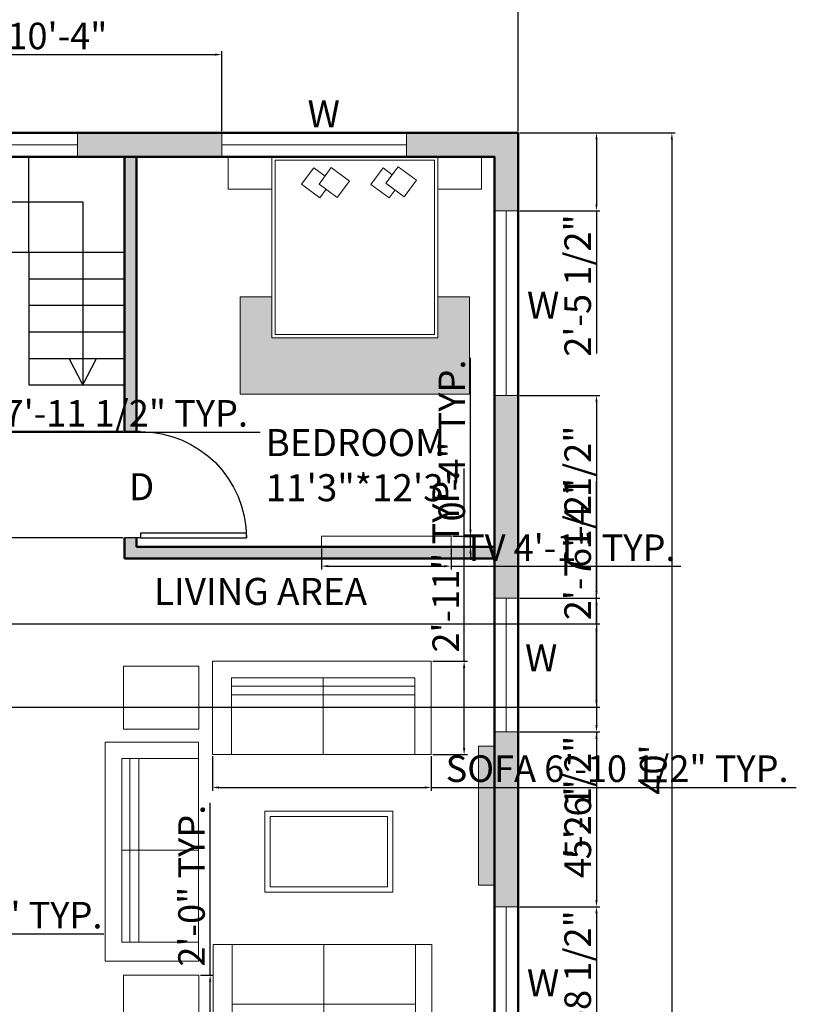
# Model space of a CAD drawing. Units: inches. Extents: x 1822 to 2392, y 2066 to 2908.
# Tile 3 of 4: x 2080 to 2373, y 2256 to 2627. Entities that reach past the tile are written whole.
import ezdxf

# ---------------------------------------------------------------- set-up
doc = ezdxf.new("R2010")
doc.units = ezdxf.units.IN
for name, color, linetype, lineweight in [('A-ANNO-DIMS', 2, 'Continuous', 18), ('A-AREA-IDEN', 83, 'Continuous', 25), ('A-EQPM-PATT', 89, 'Continuous', 13), ('A-FLOR-PATT', 9, 'Continuous', 13), ('A-FURN', 140, 'Continuous', 18), ('A-WALL-PATT', 252, 'Continuous', 13), ('BEDS', 40, 'Continuous', 18), ('DOOR', 50, 'Continuous', 25), ('SOFA', 140, 'Continuous', 18), ('STAIR', 32, 'Continuous', 25), ('TEXT', 83, 'Continuous', 25), ('TV', 89, 'Continuous', 18), ('wall', 7, 'Continuous', 50), ('WINDOW', 80, 'Continuous', 20)]:
    doc.layers.add(name, color=color, linetype=linetype, lineweight=lineweight)
doc.styles.get("Standard").update_dxf_attribs({"font": 'arial.ttf'})
doc.dimstyles.new('ISO-25', dxfattribs={"dimtxt": 10, "dimasz": 2.5, "dimexe": 1.25, "dimexo": 0.625, "dimtad": 1, "dimdec": 0, "dimlunit": 4, "dimtxsty": 'Standard', "dimcen": 2.5, "dimadec": 0, "dimazin": 0, "dimtfac": 1, "dimtdec": 0, "dimtmove": 0, "dimatfit": 3, "dimfxl": 1, "dimarcsym": 0})

# ---------------------------------------------------------------- blocks, each defined once
blk = doc.blocks.new('*U2')
for p, q in [((0, 0), (0, -6)), ((40, 0), (40, -6))]:
    blk.add_line(p, q)
blk.add_lwpolyline([(0, 0), (0, 40), (1.75, 40), (1.75, 0)], close=True)
blk.add_arc((0, 0), 40, 0, 90)
blk = doc.blocks.new('*D5')
at = {"layer": 'A-ANNO-DIMS', "color": 0, "lineweight": -2, "transparency": 16777216}
for p, q in [((1872.41, 2584.74), (1872.41, 2632.85)), ((1874.91, 2631.6), (2265.91, 2631.6)), ((2268.41, 2584.74), (2268.41, 2632.85))]:
    blk.add_line(p, q, dxfattribs=at)
at = {"layer": 'A-ANNO-DIMS', "color": 0, "transparency": 16777216}
for points in [[(1874.91, 2632.01), (1874.91, 2631.18), (1872.41, 2631.6)], [(2265.91, 2632.01), (2265.91, 2631.18), (2268.41, 2631.6)]]:
    blk.add_solid(points, dxfattribs=at)
at = {"layer": 'Defpoints', "color": 0, "transparency": 16777216}
for p in [(2268.41, 2631.6), (1872.41, 2584.12), (2268.41, 2584.12)]:
    blk.add_point(p, dxfattribs=at)
at = {"layer": 'A-ANNO-DIMS', "color": 0, "transparency": 16777216, "insert": (2070.41, 2637.33), "char_height": 10, "attachment_point": 5}
blk.add_mtext("33'", dxfattribs=at)
blk = doc.blocks.new('*D6')
at = {"layer": 'A-ANNO-DIMS', "color": 0, "lineweight": -2, "transparency": 16777216}
for p, q in [((2269.04, 2584.12), (2327.59, 2584.12)), ((2326.34, 2581.62), (2326.34, 2106.62)), ((2269.04, 2104.12), (2327.59, 2104.12))]:
    blk.add_line(p, q, dxfattribs=at)
at = {"layer": 'A-ANNO-DIMS', "color": 0, "transparency": 16777216}
for points in [[(2325.93, 2581.62), (2326.76, 2581.62), (2326.34, 2584.12)], [(2325.93, 2106.62), (2326.76, 2106.62), (2326.34, 2104.12)]]:
    blk.add_solid(points, dxfattribs=at)
at = {"layer": 'Defpoints', "color": 0, "transparency": 16777216}
for p in [(2268.41, 2584.12), (2268.41, 2104.12), (2326.34, 2104.12)]:
    blk.add_point(p, dxfattribs=at)
at = {"layer": 'A-ANNO-DIMS', "color": 0, "transparency": 16777216, "insert": (2320.61, 2344.12), "char_height": 10, "attachment_point": 5, "rotation": 90}
blk.add_mtext("40'", dxfattribs=at)
blk = doc.blocks.new('BED-DOUBLE-WITH-NIGHTSTANDS')
for p, q in [((0, -52.84), (-12, -52.84)), ((-12, -52.84), (-12, -89.47)), ((62.55, -52.84), (74.55, -52.84)), ((74.55, -52.84), (74.55, -89.47)), ((-12, -89.47), (74.55, -89.47))]:
    blk.add_line(p, q)
for points in [[(0, 0), (-16.5, 0), (-16.5, -12.19), (0, -12.19)], [(0, 0), (62.55, 0), (62.55, -68.27), (0, -68.27)], [(79.04, 0), (62.55, 0), (62.55, -12.19), (79.04, -12.19)], [(1.28, -1.28), (61.27, -1.28), (61.27, -67), (1.28, -67)], [(22.38, -4.1), (29.25, -9.19), (24.65, -15.4), (17.78, -10.31)], [(47.61, -3.78), (54.48, -8.87), (49.87, -15.08), (43, -9.99)]]:
    blk.add_lwpolyline(points, close=True)
for points in [[(20.42, -12.27), (18.06, -15.45), (11.2, -10.36), (15.8, -4.15), (20.02, -7.28)], [(46.41, -12.52), (44.19, -15.51), (37.32, -10.42), (41.93, -4.21), (45.39, -6.77)]]:
    blk.add_lwpolyline(points)
blk = doc.blocks.new('SOFA-TWO-SEAT')
for p, q in [((0, 0), (0, 35.2)), ((0, 35.2), (82.54, 35.2)), ((82.54, 35.2), (82.54, 0)), ((41.75, 28.9), (41.75, 0)), ((7.18, 25.83), (76.33, 25.83)), ((7.18, 22.51), (76.33, 22.51)), ((7.18, 0), (0, 0)), ((82.54, 0), (73.14, 0))]:
    blk.add_line(p, q)
blk.add_lwpolyline([(76.33, 0), (7.18, 0), (7.18, 28.9), (76.33, 28.9)], close=True)
blk = doc.blocks.new('WINDOW-EXT-TYPE-A')
blk.add_line((0, 4.5), (69.61, 4.5))
blk.add_lwpolyline([(0, 9), (69.61, 9), (69.61, 0), (0, 0)], close=True)
blk = doc.blocks.new('TABLE-END')
blk.add_lwpolyline([(0, 0), (28.42, 0), (28.42, 23.78), (0, 23.78)], close=True)
blk = doc.blocks.new('TV-BEDROOM-TYPE-A')
blk.add_lwpolyline([(0, 0), (48.81, 0), (48.81, 3.94), (0, 3.94)], close=True)
blk = doc.blocks.new('*D16')
at = {"layer": 'A-ANNO-DIMS', "color": 0, "lineweight": -2, "transparency": 16777216}
for p, q in [((1892.52, 2485.02), (1892.52, 2470.06)), ((1988.06, 2485.02), (1988.06, 2470.06)), ((1895.02, 2471.31), (1985.56, 2471.31)), ((1988.06, 2471.31), (2171.11, 2471.31))]:
    blk.add_line(p, q, dxfattribs=at)
at = {"layer": 'A-ANNO-DIMS', "color": 0, "transparency": 16777216}
for points in [[(1895.02, 2471.73), (1895.02, 2470.9), (1892.52, 2471.31)], [(1985.56, 2471.73), (1985.56, 2470.9), (1988.06, 2471.31)]]:
    blk.add_solid(points, dxfattribs=at)
at = {"layer": 'Defpoints', "color": 0, "transparency": 16777216}
for p in [(1892.52, 2485.65), (1988.06, 2485.65), (1988.06, 2471.31)]:
    blk.add_point(p, dxfattribs=at)
at = {"layer": 'A-ANNO-DIMS', "color": 0, "transparency": 16777216, "insert": (2080.84, 2477.11), "char_height": 10, "attachment_point": 5}
blk.add_mtext('BED GROUP 7\'-11 1/2" TYP.', dxfattribs=at)
blk = doc.blocks.new('*D18')
at = {"layer": 'A-ANNO-DIMS', "color": 0, "lineweight": -2, "transparency": 16777216}
for p, q in [((2153.07, 2349.12), (2153.07, 2336.11)), ((2235.61, 2349.12), (2235.61, 2336.11)), ((2155.57, 2337.36), (2233.11, 2337.36)), ((2235.61, 2337.36), (2373.26, 2337.36))]:
    blk.add_line(p, q, dxfattribs=at)
at = {"layer": 'A-ANNO-DIMS', "color": 0, "transparency": 16777216}
for points in [[(2155.57, 2337.78), (2155.57, 2336.95), (2153.07, 2337.36)], [(2233.11, 2337.78), (2233.11, 2336.95), (2235.61, 2337.36)]]:
    blk.add_solid(points, dxfattribs=at)
at = {"layer": 'Defpoints', "color": 0, "transparency": 16777216}
for p in [(2153.07, 2349.75), (2235.61, 2349.75), (2235.61, 2337.36)]:
    blk.add_point(p, dxfattribs=at)
at = {"layer": 'A-ANNO-DIMS', "color": 0, "transparency": 16777216, "insert": (2305.69, 2343.16), "char_height": 10, "attachment_point": 5}
blk.add_mtext('SOFA 6\'-10 1/2" TYP.', dxfattribs=at)
blk = doc.blocks.new('*D19')
at = {"layer": 'A-ANNO-DIMS', "color": 0, "lineweight": -2, "transparency": 16777216}
for p, q in [((2248, 2384.94), (2248, 2457.59)), ((2236.24, 2384.94), (2249.25, 2384.94)), ((2248, 2352.25), (2248, 2382.44)), ((2236.24, 2349.75), (2249.25, 2349.75))]:
    blk.add_line(p, q, dxfattribs=at)
at = {"layer": 'A-ANNO-DIMS', "color": 0, "transparency": 16777216}
for points in [[(2247.58, 2382.44), (2248.41, 2382.44), (2248, 2384.94)], [(2247.58, 2352.25), (2248.41, 2352.25), (2248, 2349.75)]]:
    blk.add_solid(points, dxfattribs=at)
at = {"layer": 'Defpoints', "color": 0, "transparency": 16777216}
for p in [(2235.61, 2384.94), (2248, 2384.94), (2235.61, 2349.75)]:
    blk.add_point(p, dxfattribs=at)
at = {"layer": 'A-ANNO-DIMS', "color": 0, "transparency": 16777216, "insert": (2242.35, 2422.51), "char_height": 10, "attachment_point": 5, "rotation": 90}
blk.add_mtext('2\'-11" TYP.', dxfattribs=at)
blk = doc.blocks.new('*D23')
at = {"layer": 'A-ANNO-DIMS', "color": 0, "lineweight": -2, "transparency": 16777216}
for p, q in [((2004.74, 2284.62), (2004.74, 2280.89)), ((2016.41, 2284.62), (2016.41, 2280.89)), ((2007.24, 2282.14), (2013.91, 2282.14)), ((2016.41, 2282.14), (2112.19, 2282.14))]:
    blk.add_line(p, q, dxfattribs=at)
at = {"layer": 'A-ANNO-DIMS', "color": 0, "transparency": 16777216}
for points in [[(2007.24, 2282.56), (2007.24, 2281.73), (2004.74, 2282.14)], [(2013.91, 2282.56), (2013.91, 2281.73), (2016.41, 2282.14)]]:
    blk.add_solid(points, dxfattribs=at)
at = {"layer": 'Defpoints', "color": 0, "transparency": 16777216}
for p in [(2004.74, 2285.25), (2016.41, 2285.25), (2016.41, 2282.14)]:
    blk.add_point(p, dxfattribs=at)
at = {"layer": 'A-ANNO-DIMS', "color": 0, "transparency": 16777216, "insert": (2065.55, 2287.94), "char_height": 10, "attachment_point": 5}
blk.add_mtext('0\'-11 1/2" TYP.', dxfattribs=at)
blk = doc.blocks.new('*D24')
at = {"layer": 'A-ANNO-DIMS', "color": 0, "lineweight": -2, "transparency": 16777216}
for p, q in [((2119.55, 2242.25), (2119.55, 2237.36)), ((2147.97, 2242.25), (2147.97, 2237.36)), ((2122.05, 2238.61), (2145.47, 2238.61)), ((2147.97, 2238.61), (2316.96, 2238.61))]:
    blk.add_line(p, q, dxfattribs=at)
at = {"layer": 'A-ANNO-DIMS', "color": 0, "transparency": 16777216}
for points in [[(2122.05, 2239.03), (2122.05, 2238.2), (2119.55, 2238.61)], [(2145.47, 2239.03), (2145.47, 2238.2), (2147.97, 2238.61)]]:
    blk.add_solid(points, dxfattribs=at)
at = {"layer": 'Defpoints', "color": 0, "transparency": 16777216}
for p in [(2119.55, 2242.88), (2147.97, 2242.88), (2147.97, 2238.61)]:
    blk.add_point(p, dxfattribs=at)
at = {"layer": 'A-ANNO-DIMS', "color": 0, "transparency": 16777216, "insert": (2233.72, 2244.41), "char_height": 10, "attachment_point": 5}
blk.add_mtext('END TABLE 2\'-4 1/2" TYP.', dxfattribs=at)
blk = doc.blocks.new('*D25')
at = {"layer": 'A-ANNO-DIMS', "color": 0, "lineweight": -2, "transparency": 16777216}
for p, q in [((2152.23, 2266.66), (2152.23, 2331.53)), ((2148.59, 2266.66), (2153.48, 2266.66)), ((2152.23, 2245.38), (2152.23, 2264.16)), ((2148.59, 2242.88), (2153.48, 2242.88))]:
    blk.add_line(p, q, dxfattribs=at)
at = {"layer": 'A-ANNO-DIMS', "color": 0, "transparency": 16777216}
for points in [[(2151.81, 2264.16), (2152.65, 2264.16), (2152.23, 2266.66)], [(2151.81, 2245.38), (2152.65, 2245.38), (2152.23, 2242.88)]]:
    blk.add_solid(points, dxfattribs=at)
at = {"layer": 'Defpoints', "color": 0, "transparency": 16777216}
for p in [(2147.97, 2266.66), (2152.23, 2266.66), (2147.97, 2242.88)]:
    blk.add_point(p, dxfattribs=at)
at = {"layer": 'A-ANNO-DIMS', "color": 0, "transparency": 16777216, "insert": (2146.5, 2300.35), "char_height": 10, "attachment_point": 5, "rotation": 90}
blk.add_mtext('2\'-0" TYP.', dxfattribs=at)
blk = doc.blocks.new('*D26')
at = {"layer": 'A-ANNO-DIMS', "color": 0, "lineweight": -2, "transparency": 16777216}
for p, q in [((2194.25, 2427.49), (2194.25, 2419.55)), ((2243.06, 2427.49), (2243.06, 2419.55)), ((2196.75, 2420.8), (2240.56, 2420.8)), ((2243.06, 2420.8), (2329.75, 2420.8))]:
    blk.add_line(p, q, dxfattribs=at)
at = {"layer": 'A-ANNO-DIMS', "color": 0, "transparency": 16777216}
for points in [[(2196.75, 2421.21), (2196.75, 2420.38), (2194.25, 2420.8)], [(2240.56, 2421.21), (2240.56, 2420.38), (2243.06, 2420.8)]]:
    blk.add_solid(points, dxfattribs=at)
at = {"layer": 'Defpoints', "color": 0, "transparency": 16777216}
for p in [(2194.25, 2428.12), (2243.06, 2428.12), (2243.06, 2420.8)]:
    blk.add_point(p, dxfattribs=at)
at = {"layer": 'A-ANNO-DIMS', "color": 0, "transparency": 16777216, "insert": (2287.66, 2426.44), "char_height": 10, "attachment_point": 5}
blk.add_mtext('TV 4\'-1" TYP.', dxfattribs=at)
blk = doc.blocks.new('*D27')
at = {"layer": 'A-ANNO-DIMS', "color": 0, "lineweight": -2, "transparency": 16777216}
for p, q in [((2250.38, 2434.56), (2250.38, 2499.26)), ((2243.69, 2432.06), (2251.63, 2432.06)), ((2250.38, 2428.12), (2250.38, 2432.06)), ((2243.69, 2428.12), (2251.63, 2428.12)), ((2250.38, 2425.62), (2250.38, 2423.12))]:
    blk.add_line(p, q, dxfattribs=at)
at = {"layer": 'A-ANNO-DIMS', "color": 0, "transparency": 16777216}
for points in [[(2249.97, 2434.56), (2250.8, 2434.56), (2250.38, 2432.06)], [(2249.97, 2425.62), (2250.8, 2425.62), (2250.38, 2428.12)]]:
    blk.add_solid(points, dxfattribs=at)
at = {"layer": 'Defpoints', "color": 0, "transparency": 16777216}
for p in [(2243.06, 2432.06), (2250.38, 2432.06), (2243.06, 2428.12)]:
    blk.add_point(p, dxfattribs=at)
at = {"layer": 'A-ANNO-DIMS', "color": 0, "transparency": 16777216, "insert": (2244.65, 2468.16), "char_height": 10, "attachment_point": 5, "rotation": 90}
blk.add_mtext('0\'-4" TYP.', dxfattribs=at)
blk = doc.blocks.new('*D30')
at = {"layer": 'A-ANNO-DIMS', "color": 0, "lineweight": -2, "transparency": 16777216}
for p, q in [((2032.62, 2584.74), (2032.62, 2614.87)), ((2035.12, 2613.62), (2154.11, 2613.62)), ((2156.61, 2584.74), (2156.61, 2614.87))]:
    blk.add_line(p, q, dxfattribs=at)
at = {"layer": 'A-ANNO-DIMS', "color": 0, "transparency": 16777216}
for points in [[(2035.12, 2614.03), (2035.12, 2613.2), (2032.62, 2613.62)], [(2154.11, 2614.03), (2154.11, 2613.2), (2156.61, 2613.62)]]:
    blk.add_solid(points, dxfattribs=at)
at = {"layer": 'Defpoints', "color": 0, "transparency": 16777216}
for p in [(2156.61, 2613.62), (2032.62, 2584.12), (2156.61, 2584.12)]:
    blk.add_point(p, dxfattribs=at)
at = {"layer": 'A-ANNO-DIMS', "color": 0, "transparency": 16777216, "insert": (2094.62, 2619.35), "char_height": 10, "attachment_point": 5}
blk.add_mtext('10\'-4"', dxfattribs=at)
blk = doc.blocks.new('*D31')
at = {"layer": 'A-ANNO-DIMS', "color": 0, "lineweight": -2, "transparency": 16777216}
for p, q in [((2269.04, 2584.12), (2299.16, 2584.12)), ((2297.91, 2581.62), (2297.91, 2557.23)), ((2269.04, 2554.73), (2299.16, 2554.73)), ((2297.91, 2554.73), (2297.91, 2500.93))]:
    blk.add_line(p, q, dxfattribs=at)
at = {"layer": 'A-ANNO-DIMS', "color": 0, "transparency": 16777216}
for points in [[(2297.5, 2581.62), (2298.33, 2581.62), (2297.91, 2584.12)], [(2297.5, 2557.23), (2298.33, 2557.23), (2297.91, 2554.73)]]:
    blk.add_solid(points, dxfattribs=at)
at = {"layer": 'Defpoints', "color": 0, "transparency": 16777216}
for p in [(2268.41, 2584.12), (2268.41, 2554.73), (2297.91, 2554.73)]:
    blk.add_point(p, dxfattribs=at)
at = {"layer": 'A-ANNO-DIMS', "color": 0, "transparency": 16777216, "insert": (2292.12, 2526.58), "char_height": 10, "attachment_point": 5, "rotation": 90}
blk.add_mtext('2\'-5 1/2"', dxfattribs=at)
blk = doc.blocks.new('*D32')
at = {"layer": 'A-ANNO-DIMS', "color": 0, "lineweight": -2, "transparency": 16777216}
for p, q in [((2269.04, 2485.12), (2299.16, 2485.12)), ((2297.91, 2482.62), (2297.91, 2411.26)), ((2269.04, 2408.76), (2299.16, 2408.76))]:
    blk.add_line(p, q, dxfattribs=at)
at = {"layer": 'A-ANNO-DIMS', "color": 0, "transparency": 16777216}
for points in [[(2297.5, 2482.62), (2298.33, 2482.62), (2297.91, 2485.12)], [(2297.5, 2411.26), (2298.33, 2411.26), (2297.91, 2408.76)]]:
    blk.add_solid(points, dxfattribs=at)
at = {"layer": 'Defpoints', "color": 0, "transparency": 16777216}
for p in [(2268.41, 2485.12), (2268.41, 2408.76), (2297.91, 2408.76)]:
    blk.add_point(p, dxfattribs=at)
at = {"layer": 'A-ANNO-DIMS', "color": 0, "transparency": 16777216, "insert": (2292.12, 2446.94), "char_height": 10, "attachment_point": 5, "rotation": 90}
blk.add_mtext('6\'-4 1/2"', dxfattribs=at)
blk = doc.blocks.new('*D33')
at = {"layer": 'A-ANNO-DIMS', "color": 0, "lineweight": -2, "transparency": 16777216}
for p, q in [((2269.04, 2408.76), (2299.16, 2408.76)), ((2297.91, 2406.26), (2297.91, 2360.82)), ((2269.04, 2358.32), (2299.16, 2358.32)), ((2297.91, 2358.32), (2297.91, 2304.28))]:
    blk.add_line(p, q, dxfattribs=at)
at = {"layer": 'A-ANNO-DIMS', "color": 0, "transparency": 16777216}
for points in [[(2297.5, 2406.26), (2298.33, 2406.26), (2297.91, 2408.76)], [(2297.5, 2360.82), (2298.33, 2360.82), (2297.91, 2358.32)]]:
    blk.add_solid(points, dxfattribs=at)
at = {"layer": 'Defpoints', "color": 0, "transparency": 16777216}
for p in [(2268.41, 2408.76), (2268.41, 2358.32), (2297.91, 2358.32)]:
    blk.add_point(p, dxfattribs=at)
at = {"layer": 'A-ANNO-DIMS', "color": 0, "transparency": 16777216, "insert": (2292.12, 2330.05), "char_height": 10, "attachment_point": 5, "rotation": 90}
blk.add_mtext('4\'-2 1/2"', dxfattribs=at)
blk = doc.blocks.new('*D34')
at = {"layer": 'A-ANNO-DIMS', "color": 0, "lineweight": -2, "transparency": 16777216}
for p, q in [((2269.04, 2358.32), (2299.16, 2358.32)), ((2297.91, 2355.82), (2297.91, 2294.9)), ((2269.04, 2292.4), (2299.16, 2292.4))]:
    blk.add_line(p, q, dxfattribs=at)
at = {"layer": 'A-ANNO-DIMS', "color": 0, "transparency": 16777216}
for points in [[(2297.5, 2355.82), (2298.33, 2355.82), (2297.91, 2358.32)], [(2297.5, 2294.9), (2298.33, 2294.9), (2297.91, 2292.4)]]:
    blk.add_solid(points, dxfattribs=at)
at = {"layer": 'Defpoints', "color": 0, "transparency": 16777216}
for p in [(2268.41, 2358.32), (2268.41, 2292.4), (2297.91, 2292.4)]:
    blk.add_point(p, dxfattribs=at)
at = {"layer": 'A-ANNO-DIMS', "color": 0, "transparency": 16777216, "insert": (2292.18, 2325.36), "char_height": 10, "attachment_point": 5, "rotation": 90}
blk.add_mtext('5\'-6"', dxfattribs=at)
blk = doc.blocks.new('*D35')
at = {"layer": 'A-ANNO-DIMS', "color": 0, "lineweight": -2, "transparency": 16777216}
for p, q in [((2269.04, 2292.4), (2299.16, 2292.4)), ((2297.91, 2289.9), (2297.91, 2238.6)), ((2269.04, 2236.1), (2299.16, 2236.1))]:
    blk.add_line(p, q, dxfattribs=at)
at = {"layer": 'A-ANNO-DIMS', "color": 0, "transparency": 16777216}
for points in [[(2297.5, 2289.9), (2298.33, 2289.9), (2297.91, 2292.4)], [(2297.5, 2238.6), (2298.33, 2238.6), (2297.91, 2236.1)]]:
    blk.add_solid(points, dxfattribs=at)
at = {"layer": 'Defpoints', "color": 0, "transparency": 16777216}
for p in [(2268.41, 2292.4), (2268.41, 2236.1), (2297.91, 2236.1)]:
    blk.add_point(p, dxfattribs=at)
at = {"layer": 'A-ANNO-DIMS', "color": 0, "transparency": 16777216, "insert": (2292.12, 2264.25), "char_height": 10, "attachment_point": 5, "rotation": 90}
blk.add_mtext('4\'-8 1/2"', dxfattribs=at)
blk = doc.blocks.new('*D43')
at = {"layer": 'A-ANNO-DIMS', "color": 0, "lineweight": -2, "transparency": 16777216}
for p, q in [((2119.29, 2471.52), (1841.66, 2471.52)), ((1842.91, 2434.02), (1842.91, 2469.02)), ((2119.29, 2431.52), (1841.66, 2431.52))]:
    blk.add_line(p, q, dxfattribs=at)
at = {"layer": 'A-ANNO-DIMS', "color": 0, "transparency": 16777216}
for points in [[(1842.5, 2469.02), (1843.33, 2469.02), (1842.91, 2471.52)], [(1842.5, 2434.02), (1843.33, 2434.02), (1842.91, 2431.52)]]:
    blk.add_solid(points, dxfattribs=at)
at = {"layer": 'Defpoints', "color": 0, "transparency": 16777216}
for p in [(1842.91, 2471.52), (2119.91, 2471.52), (2119.91, 2431.52)]:
    blk.add_point(p, dxfattribs=at)
at = {"layer": 'A-ANNO-DIMS', "color": 0, "transparency": 16777216, "insert": (1837.18, 2451.52), "char_height": 10, "attachment_point": 5, "rotation": 90}
blk.add_mtext('3\'-4"', dxfattribs=at)
blk = doc.blocks.new('*D44')
at = {"layer": 'A-ANNO-DIMS', "color": 0, "lineweight": -2, "transparency": 16777216}
for p, q in [((2297.91, 2399.09), (2297.91, 2452.89)), ((1974.54, 2399.09), (2299.16, 2399.09)), ((2297.91, 2370.08), (2297.91, 2396.59)), ((1974.54, 2367.58), (2299.16, 2367.58))]:
    blk.add_line(p, q, dxfattribs=at)
at = {"layer": 'A-ANNO-DIMS', "color": 0, "transparency": 16777216}
for points in [[(2297.5, 2396.59), (2298.33, 2396.59), (2297.91, 2399.09)], [(2297.5, 2370.08), (2298.33, 2370.08), (2297.91, 2367.58)]]:
    blk.add_solid(points, dxfattribs=at)
at = {"layer": 'Defpoints', "color": 0, "transparency": 16777216}
for p in [(1973.91, 2399.09), (2297.91, 2399.09), (1973.91, 2367.58)]:
    blk.add_point(p, dxfattribs=at)
at = {"layer": 'A-ANNO-DIMS', "color": 0, "transparency": 16777216, "insert": (2292.12, 2427.24), "char_height": 10, "attachment_point": 5, "rotation": 90}
blk.add_mtext('2\'-7 1/2"', dxfattribs=at)

msp = doc.modelspace()

# ---------------------------------------------------------------- hatches: boundary and pattern name
at = {"layer": 'A-EQPM-PATT'}
h = msp.add_hatch(color=256, dxfattribs=at)
h.dxf.hatch_style = 1
h.paths.add_polyline_path([(2259.41, 2352.89), (2253.4, 2352.89), (2253.4, 2300.49), (2259.41, 2300.49)])
h.paths.add_polyline_path([(1972.53, 2267.62), (1927.37, 2267.62), (1927.37, 2261.95), (1972.53, 2261.95)])
h.paths.add_polyline_path([(1953.54, 2432.06), (1904.73, 2432.06), (1904.73, 2428.12), (1953.54, 2428.12)])
at = {"layer": 'A-FLOR-PATT'}
h = msp.add_hatch(dxfattribs=at)
h.set_pattern_fill('ANSI36', color=256)
h.paths.add_polyline_path([(1983.57, 2522.27), (1971.57, 2522.27), (1971.57, 2506.84), (1909.02, 2506.84), (1909.02, 2522.27), (1897.02, 2522.27), (1897.02, 2485.65), (1983.57, 2485.65)])
h.paths.add_polyline_path([(1988.24, 2202.59), (1901.7, 2202.59), (1901.7, 2165.96), (1913.7, 2165.96), (1913.7, 2181.39), (1976.24, 2181.39), (1976.24, 2165.96), (1988.24, 2165.96)])
h.paths.add_polyline_path([(2250.08, 2522.27), (2238.08, 2522.27), (2238.08, 2506.84), (2175.53, 2506.84), (2175.53, 2522.27), (2163.53, 2522.27), (2163.53, 2485.65), (2250.08, 2485.65)])
at = {"layer": 'A-WALL-PATT'}
h = msp.add_hatch(color=256, dxfattribs=at)
h.dxf.hatch_style = 1
h.paths.add_polyline_path([(2032.62, 2584.12), (1982.01, 2584.12), (1982.01, 2575.12), (1988.06, 2575.12), (2016.41, 2575.12), (2032.62, 2575.12)], flags=17)
h.paths.add_polyline_path([(2156.61, 2584.12), (2102.23, 2584.12), (2102.23, 2575.12), (2119.91, 2575.12), (2156.61, 2575.12)], flags=17)
h.paths.add_polyline_path([(1914.42, 2104.12), (1914.42, 2113.12), (1881.41, 2113.12), (1881.41, 2575.12), (1912.4, 2575.12), (1912.4, 2584.12), (1872.41, 2584.12), (1872.41, 2104.12)])
h.paths.add_polyline_path([(2268.41, 2129.27), (2259.41, 2129.27), (2259.41, 2113.12), (2224.8, 2113.12), (2224.8, 2104.12), (2268.41, 2104.12)])
h.paths.add_polyline_path([(2268.41, 2236.1), (2259.41, 2236.1), (2259.41, 2198.88), (2268.41, 2198.88)])
h.paths.add_polyline_path([(2268.41, 2358.32), (2259.41, 2358.32), (2259.41, 2292.4), (2268.41, 2292.4)])
h.paths.add_polyline_path([(2259.41, 2554.73), (2268.41, 2554.73), (2268.41, 2584.12), (2226.22, 2584.12), (2226.22, 2575.12), (2259.41, 2575.12)])
h.paths.add_polyline_path([(2268.41, 2485.12), (2259.41, 2485.12), (2259.41, 2408.76), (2268.41, 2408.76)])
h.paths.add_polyline_path([(2020.91, 2104.12), (2020.91, 2113.12), (1984.03, 2113.12), (1984.03, 2104.12)])
h.paths.add_polyline_path([(2119.91, 2113.12), (2119.91, 2104.12), (2155.19, 2104.12), (2155.19, 2113.12)])
h = msp.add_hatch(color=256, dxfattribs=at)
h.dxf.hatch_style = 1
h.paths.add_polyline_path([(2124.41, 2575.12), (2119.91, 2575.12), (2119.91, 2471.52), (2124.41, 2471.52)])
h.paths.add_polyline_path([(2020.91, 2575.12), (2016.41, 2575.12), (2016.41, 2471.18), (2020.91, 2471.18)])
h.paths.add_polyline_path([(2259.41, 2428.12), (2124.41, 2428.12), (2124.41, 2431.52), (2119.91, 2431.52), (2119.91, 2423.62), (2259.41, 2423.62)])
h.paths.add_polyline_path([(2020.91, 2363.62), (2016.41, 2363.62), (2015.38, 2363.62), (2015.38, 2359.12), (2016.41, 2359.12), (2016.41, 2272.12), (1945.91, 2272.12), (1945.91, 2305.88), (1941.41, 2305.88), (1941.41, 2272.12), (1923.14, 2272.12), (1923.14, 2267.62), (2016.41, 2267.62), (2016.41, 2261.67), (2020.91, 2261.67), (2020.91, 2267.62)])
h.paths.add_polyline_path([(2259.41, 2213.62), (2168.4, 2213.62), (2168.4, 2209.12), (2259.41, 2209.12)])
h.paths.add_polyline_path([(2124.41, 2209.12), (2128.4, 2209.12), (2128.4, 2213.62), (2119.91, 2213.62), (2119.91, 2113.12), (2124.41, 2113.12), (2124.41, 2137.12)])
h.paths.add_polyline_path([(2020.91, 2221.67), (2016.41, 2221.67), (2016.41, 2113.12), (2020.91, 2113.12), (2020.91, 2137.12)])
h.paths.add_polyline_path([(2034.48, 2141.62), (2020.91, 2141.62), (2020.91, 2137.12), (2034.48, 2137.12)])
h.paths.add_polyline_path([(2119.91, 2141.62), (2102.28, 2141.62), (2102.28, 2137.12), (2119.91, 2137.12)])
h.paths.add_polyline_path([(1973.91, 2423.62), (1969.41, 2423.62), (1969.41, 2399.09), (1973.91, 2399.09)])

# ---------------------------------------------------------------- linework, layer by layer
at = {"layer": 'A-FURN'}
for points in [[(2172.84, 2297.89), (2221.15, 2297.89), (2221.15, 2328.42), (2172.84, 2328.42)], [(2174.84, 2299.89), (2219.15, 2299.89), (2219.15, 2326.42), (2174.84, 2326.42)]]:
    msp.add_lwpolyline(points, close=True, dxfattribs=at)
at = {"layer": 'STAIR'}
for p, q in [((2119.91, 2575.12), (2083.91, 2575.12)), ((2083.91, 2539.12), (2083.91, 2575.12)), ((2036.89, 2558.17), (2104.24, 2558.17)), ((2104.24, 2558.17), (2104.24, 2489.12)), ((2056.91, 2539.12), (2083.91, 2539.12)), ((2083.91, 2539.12), (2083.91, 2489.12)), ((2083.91, 2539.12), (2119.91, 2539.12)), ((2083.91, 2529.12), (2119.91, 2529.12)), ((2083.91, 2519.12), (2119.91, 2519.12)), ((2083.91, 2509.12), (2119.91, 2509.12)), ((2083.91, 2499.12), (2119.91, 2499.12)), ((2104.24, 2489.12), (2099.09, 2499.12)), ((2104.24, 2489.12), (2109.38, 2499.12)), ((2083.91, 2489.12), (2119.91, 2489.12))]:
    msp.add_line(p, q, dxfattribs=at)
at = {"layer": 'TV'}
msp.add_lwpolyline([(2259.41, 2352.89), (2253.4, 2352.89), (2253.4, 2300.49), (2259.41, 2300.49)], close=True, dxfattribs=at)
at = {"layer": 'wall'}
for p, q in [((2119.91, 2575.12), (2119.91, 2471.52)), ((2259.41, 2575.12), (2124.41, 2575.12)), ((2124.41, 2575.12), (2124.41, 2471.52)), ((2119.91, 2431.52), (2119.91, 2423.62)), ((2124.41, 2431.52), (2124.41, 2428.12)), ((2124.41, 2428.12), (2259.41, 2428.12)), ((2119.91, 2423.62), (2259.41, 2423.62))]:
    msp.add_line(p, q, dxfattribs=at)
for points in [[(2119.91, 2104.12), (2268.41, 2104.12), (2268.41, 2584.12), (1872.41, 2584.12), (1872.41, 2104.12), (2020.91, 2104.12)], [(2119.91, 2113.12), (2259.41, 2113.12), (2259.41, 2575.12), (1881.41, 2575.12), (1881.41, 2113.12), (2020.91, 2113.12)]]:
    msp.add_lwpolyline(points, dxfattribs=at)
at = {"layer": 'WINDOW'}
for p, q in [((2263.91, 2408.76), (2263.91, 2358.32)), ((2263.91, 2292.4), (2263.91, 2236.1))]:
    msp.add_line(p, q, dxfattribs=at)
for points in [[(2268.41, 2408.76), (2268.41, 2358.32), (2259.41, 2358.32), (2259.41, 2408.76)], [(2268.41, 2292.4), (2268.41, 2236.1), (2259.41, 2236.1), (2259.41, 2292.4)]]:
    msp.add_lwpolyline(points, close=True, dxfattribs=at)

# ---------------------------------------------------------------- block references
at = {"layer": 'A-FURN'}
for p in [(2119.55, 2359.3), (2119.55, 2242.88)]:
    msp.add_blockref('TABLE-END', p, dxfattribs=at)
at = {"layer": 'BEDS'}
msp.add_blockref('BED-DOUBLE-WITH-NIGHTSTANDS', (2175.53, 2575.12), dxfattribs=at)
at = {"layer": 'DOOR', "xscale": -1, "rotation": 270}
msp.add_blockref('*U2', (2125.91, 2431.52), dxfattribs=at)
at = {"layer": 'SOFA'}
msp.add_blockref('SOFA-TWO-SEAT', (2153.07, 2349.74), dxfattribs=at)
at = {"layer": 'SOFA', "rotation": 89.99999999999996}
msp.add_blockref('SOFA-TWO-SEAT', (2147.8, 2271.93), dxfattribs=at)
at = {"layer": 'SOFA', "extrusion": (0, 0, -1), "zscale": -1, "rotation": 180}
msp.add_blockref('SOFA-TWO-SEAT', (-2153.31, 2278.17), dxfattribs=at)
at = {"layer": 'TV'}
msp.add_blockref('TV-BEDROOM-TYPE-A', (2194.25, 2428.12), dxfattribs=at)
at = {"layer": 'WINDOW'}
for p in [(2032.62, 2575.12), (2156.61, 2575.12)]:
    msp.add_blockref('WINDOW-EXT-TYPE-A', p, dxfattribs=at)
at = {"layer": 'WINDOW', "rotation": 269.9999999999973}
msp.add_blockref('WINDOW-EXT-TYPE-A', (2259.41, 2554.73), dxfattribs=at)

# ---------------------------------------------------------------- texts
at = {"layer": 'A-AREA-IDEN', "char_height": 10.1937, "attachment_point": 1}
for s, insert in [('BEDROOM\\P11\'3"*12\'3"', (2173.15, 2472.46)), ('LIVING AREA', (2131.02, 2416.36))]:
    msp.add_mtext_dynamic_manual_height_columns(s, width=251.9343, gutter_width=50.97, heights=[0], dxfattribs=dict(at, insert=insert))
at = {"layer": 'TEXT', "char_height": 10.19, "attachment_point": 1}
for s, insert in [('W', (2188.96, 2596.38)), ('W', (2271.69, 2524.28)), ('D', (2121.59, 2455.84)), ('W', (2270.97, 2391.35)), ('W', (2271.67, 2268.87))]:
    msp.add_mtext_dynamic_manual_height_columns(s, width=251.9343, gutter_width=50.97, heights=[0], dxfattribs=dict(at, insert=insert))

# ---------------------------------------------------------------- dimensions: what is measured, and where the dimension line sits
at = {"layer": 'A-ANNO-DIMS'}
for base, p1, p2, override, picture, middle in [((2268.41, 2631.6), (1872.41, 2584.12), (2268.41, 2584.12), {"dimclrd": 0, "dimclre": 0, "dimclrt": 0}, '*D5', (2070.41, 2637.33)), ((2156.61, 2613.62), (2032.62, 2584.12), (2156.61, 2584.12), {"dimdec": 1, "dimlfac": 1, "dimrnd": 0, "dimzin": 1, "dimdsep": 46, "dimlunit": 4, "dimfrac": 2}, '*D30', (2094.62, 2619.35))]:
    dim = msp.add_linear_dim(base=base, p1=p1, p2=p2, dimstyle='ISO-25', override=override, dxfattribs=at)
    dim.commit()
    dim.dimension.update_dxf_attribs({"geometry": picture, "text_midpoint": middle})
for base, p1, p2, override, picture, middle in [((2326.34, 2104.12), (2268.41, 2584.12), (2268.41, 2104.12), {"dimclrd": 0, "dimclre": 0, "dimclrt": 0}, '*D6', (2320.61, 2344.12)), ((2297.91, 2554.73), (2268.41, 2584.12), (2268.41, 2554.73), {"dimdec": 1, "dimlfac": 1, "dimrnd": 0, "dimzin": 1, "dimdsep": 46, "dimlunit": 4, "dimfrac": 2}, '*D31', (2292.12, 2526.58)), ((2297.91, 2408.76), (2268.41, 2485.12), (2268.41, 2408.76), {"dimdec": 1, "dimlfac": 1, "dimrnd": 0, "dimzin": 1, "dimdsep": 46, "dimlunit": 4, "dimfrac": 2}, '*D32', (2292.12, 2446.94)), ((1842.91, 2471.52), (2119.91, 2431.52), (2119.91, 2471.52), {"dimdec": 1, "dimlfac": 1, "dimrnd": 0, "dimzin": 1, "dimdsep": 46, "dimlunit": 4, "dimfrac": 2}, '*D43', (1837.18, 2451.52)), ((2297.91, 2399.09), (1973.91, 2367.58), (1973.91, 2399.09), {"dimdec": 1, "dimlfac": 1, "dimrnd": 0, "dimzin": 1, "dimdsep": 46, "dimlunit": 4, "dimfrac": 2}, '*D44', (2292.12, 2427.24)), ((2297.91, 2358.32), (2268.41, 2408.76), (2268.41, 2358.32), {"dimdec": 1, "dimlfac": 1, "dimrnd": 0, "dimzin": 1, "dimdsep": 46, "dimlunit": 4, "dimfrac": 2}, '*D33', (2292.12, 2330.05)), ((2297.91, 2292.4), (2268.41, 2358.32), (2268.41, 2292.4), {"dimdec": 1, "dimlfac": 1, "dimrnd": 0, "dimzin": 1, "dimdsep": 46, "dimlunit": 4, "dimfrac": 2}, '*D34', (2292.18, 2325.36)), ((2297.91, 2236.1), (2268.41, 2292.4), (2268.41, 2236.1), {"dimdec": 1, "dimlfac": 1, "dimrnd": 0, "dimzin": 1, "dimdsep": 46, "dimlunit": 4, "dimfrac": 2}, '*D35', (2292.12, 2264.25))]:
    dim = msp.add_linear_dim(base=base, p1=p1, p2=p2, angle=90, dimstyle='ISO-25', override=override, dxfattribs=at)
    dim.commit()
    dim.dimension.update_dxf_attribs({"geometry": picture, "text_midpoint": middle})
for base, p1, p2, text, picture, middle in [((1988.06, 2471.31), (1892.52, 2485.65), (1988.06, 2485.65), 'BED GROUP <> TYP.', '*D16', (2080.84, 2477.11)), ((2243.06, 2420.8), (2194.25, 2428.12), (2243.06, 2428.12), 'TV <> TYP.', '*D26', (2287.66, 2426.44)), ((2235.61, 2337.36), (2153.07, 2349.75), (2235.61, 2349.75), 'SOFA <> TYP.', '*D18', (2305.69, 2343.16)), ((2016.41, 2282.14), (2004.74, 2285.25), (2016.41, 2285.25), '<> TYP.', '*D23', (2065.55, 2287.94)), ((2147.97, 2238.61), (2119.55, 2242.88), (2147.97, 2242.88), 'END TABLE <> TYP.', '*D24', (2233.72, 2244.41))]:
    dim = msp.add_linear_dim(base=base, p1=p1, p2=p2, text=text, dimstyle='ISO-25', override={"dimdec": 1, "dimlfac": 1, "dimrnd": 0, "dimzin": 1, "dimdsep": 46, "dimlunit": 4, "dimfrac": 2}, dxfattribs=at)
    dim.commit()
    dim.dimension.update_dxf_attribs({"geometry": picture, "text_midpoint": middle})
for base, p1, p2, picture, middle in [((2250.38, 2432.06), (2243.06, 2428.12), (2243.06, 2432.06), '*D27', (2244.65, 2468.16)), ((2248, 2384.94), (2235.61, 2349.75), (2235.61, 2384.94), '*D19', (2242.35, 2422.51)), ((2152.23, 2266.66), (2147.97, 2242.88), (2147.97, 2266.66), '*D25', (2146.5, 2300.35))]:
    dim = msp.add_linear_dim(base=base, p1=p1, p2=p2, angle=90, text='<> TYP.', dimstyle='ISO-25', override={"dimdec": 1, "dimlfac": 1, "dimrnd": 0, "dimzin": 1, "dimdsep": 46, "dimlunit": 4, "dimfrac": 2}, dxfattribs=at)
    dim.commit()
    dim.dimension.update_dxf_attribs({"geometry": picture, "text_midpoint": middle})

doc.saveas('drawing.dxf')
